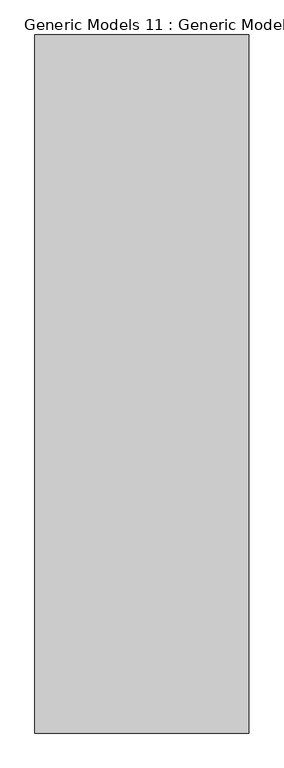
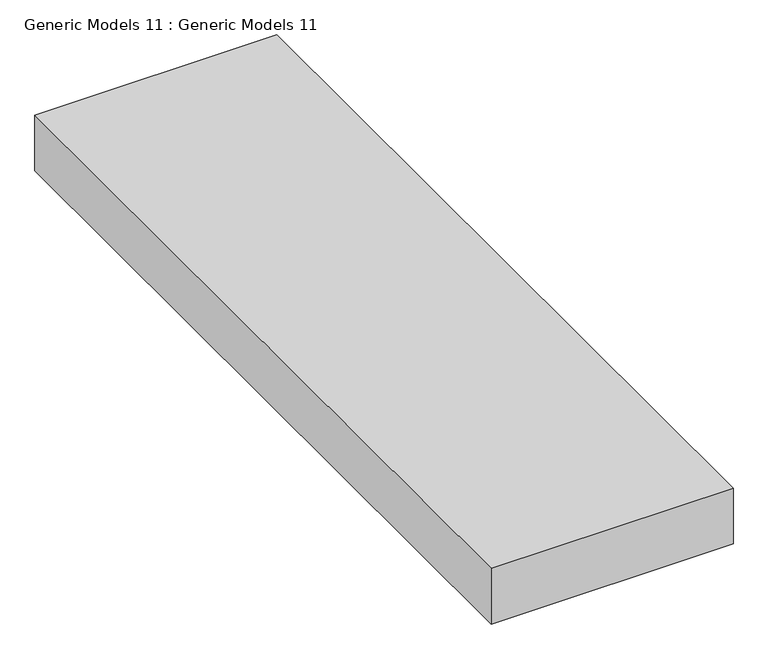
"""IFC4 building model written with IfcOpenShell, lengths in millimetres: proxy geometry, Generic Models 11 : Generic Models 11."""

from ifc_helpers import new_model, si_unit, frame, origin, place, context, project, spatial, polyline, outline, extrude, source, transform, mapped, element, save


def generic_models_11_generic_models_11_b310268c(model_context):
    return source(origin(), model_context, "Body", "SweptSolid", [
        extrude(outline(polyline([(-16847.8054227, -10247.2773911), (-16847.8054227, -8207.5302573), (-16223.0859258, -8207.5302573), (-16223.0859258, -10247.2773911), (-16847.8054227, -10247.2773911)])), frame((0.0, 0.0, 2585.6396252), z_axis=(0.0, 0.0, 1.0), x_axis=(1.0, 0.0, 0.0)), (0.0, 0.0, 1.0), 152.4),
    ])


if __name__ == "__main__":
    model = new_model("IFC4")
    model_context = context("Model", 3, world=origin())
    ifc_project = project(units=[si_unit("LENGTHUNIT", "METRE", prefix="MILLI")], contexts=[model_context])
    site = spatial("IfcSite", under=ifc_project)
    building = spatial("IfcBuilding", under=site)
    placement = place(None, origin())
    generic_models_11_generic_models_11_shape = generic_models_11_generic_models_11_b310268c(model_context)
    element("IfcBuildingElementProxy", 1, Name="Generic Models 11 : Generic Models 11", ObjectType="Generic Models 11 : Generic Models 11", at=placement, inside=building, context=model_context, shape_type="MappedRepresentation", body=[
        mapped(generic_models_11_generic_models_11_shape, transform((0.0, 0.0, 0.0), x_axis=(1.0, 0.0, 0.0), y_axis=(0.0, 1.0, 0.0), z_axis=(0.0, 0.0, 1.0))),
    ])
    save(model, "model.ifc")
